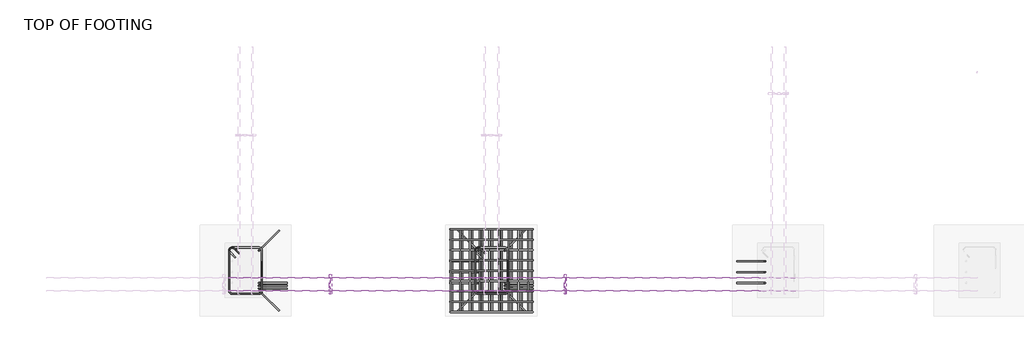
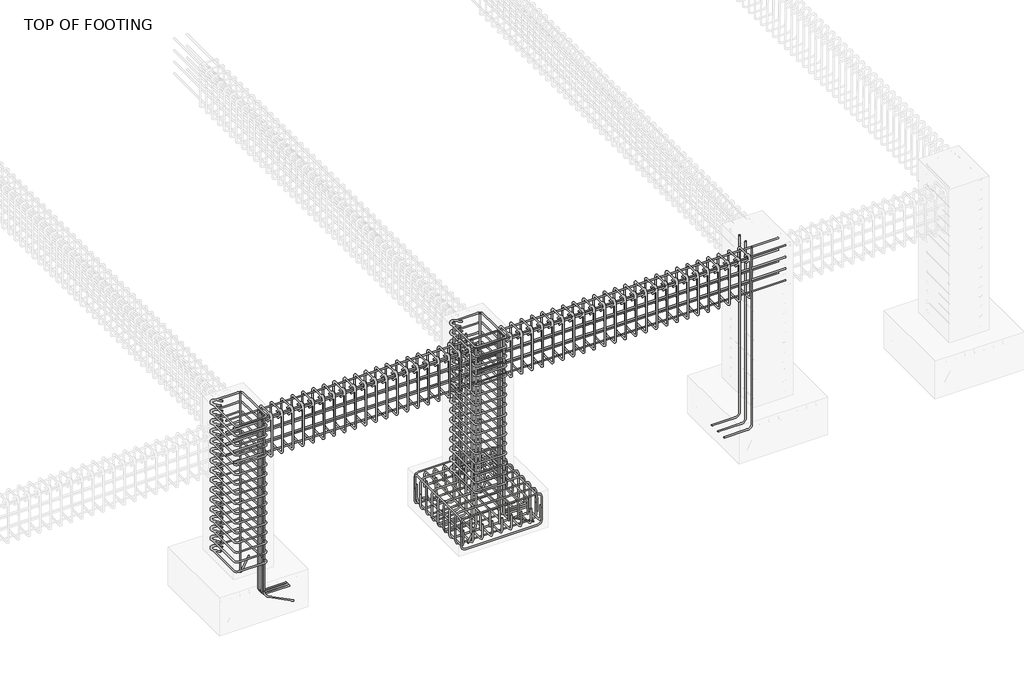
# One storey, part 3 of 9: 22 reinforcing bars.
"""IFC4 building model written with IfcOpenShell, lengths in millimetres."""

from ifc_helpers import new_model, si_unit, point, frame, origin, place, context, project, spatial, polyline, circle_curve, trimmed, segment, composite_curve, source, transform, mapped, element, save
from ifc_brep_helpers import swept_disk

model = new_model("IFC4")

# Units and contexts
model_context = context("Model", 3, world=origin())
ifc_project = project(units=[si_unit("LENGTHUNIT", "METRE", prefix="MILLI")], contexts=[model_context])

# Site, building, storey
site = spatial("IfcSite", under=ifc_project)
building = spatial("IfcBuilding", under=site)
storey = spatial("IfcBuildingStorey", under=building, Name="TOP OF FOOTING", Elevation=-1828.8)

# Reinforcing bars
placement = place(None, origin())
reinforcing_bar_shape = source(origin(), model_context, "Body", "SolidModel", [
    swept_disk(composite_curve([segment(polyline([(-4629.6174526, -598.6824927, -2052.8356656), (-4629.6174526, -598.6824927, -2200.1356656)]), True, "CONTINUOUS"), segment(trimmed(circle_curve(frame((-4675.9674526, -598.6824927, -2200.1356656), z_axis=(0.0, 1.0, 0.0), x_axis=(46.349999999999454, 0.0, 0.0)), 46.35), [point((-4629.6174526, -598.6824927, -2200.1356656))], [point((-4675.9674526, -598.6824927, -2246.4856656))], True, "CARTESIAN"), True, "CONTINUOUS"), segment(polyline([(-4675.9674526, -598.6824927, -2246.4856656), (-5490.5674526, -598.6824927, -2246.4856656)]), True, "CONTINUOUS"), segment(trimmed(circle_curve(frame((-5490.5674526, -598.6824927, -2200.1356656), z_axis=(0.0, 1.0, 0.0), x_axis=(0.0, 0.0, -46.350000000000364)), 46.35), [point((-5490.5674526, -598.6824927, -2246.4856656))], [point((-5536.9174526, -598.6824927, -2200.1356656))], True, "CARTESIAN"), True, "CONTINUOUS"), segment(polyline([(-5536.9174526, -598.6824927, -2200.1356656), (-5536.9174526, -598.6824927, -2052.8356656)]), True, "CONTINUOUS")], self_intersect=False), 6.35),
])
element("IfcReinforcingBar", 1, at=placement, inside=storey, context=model_context, shape_type="MappedRepresentation", body=[
    mapped(reinforcing_bar_shape, transform((0.0, 0.0, 0.0), x_axis=(1.0, 0.0, 0.0), y_axis=(0.0, 1.0, 0.0), z_axis=(0.0, 0.0, 1.0))),
    mapped(reinforcing_bar_shape, transform((0.0, -113.4125, 0.0), x_axis=(1.0, 0.0, 0.0), y_axis=(0.0, 1.0, 0.0), z_axis=(0.0, 0.0, 1.0))),
    mapped(reinforcing_bar_shape, transform((0.0, -226.825, 0.0), x_axis=(1.0, 0.0, 0.0), y_axis=(0.0, 1.0, 0.0), z_axis=(0.0, 0.0, 1.0))),
    mapped(reinforcing_bar_shape, transform((0.0, -340.2375, 0.0), x_axis=(1.0, 0.0, 0.0), y_axis=(0.0, 1.0, 0.0), z_axis=(0.0, 0.0, 1.0))),
    mapped(reinforcing_bar_shape, transform((0.0, -453.65, 0.0), x_axis=(1.0, 0.0, 0.0), y_axis=(0.0, 1.0, 0.0), z_axis=(0.0, 0.0, 1.0))),
    mapped(reinforcing_bar_shape, transform((0.0, -567.0625, 0.0), x_axis=(1.0, 0.0, 0.0), y_axis=(0.0, 1.0, 0.0), z_axis=(0.0, 0.0, 1.0))),
    mapped(reinforcing_bar_shape, transform((0.0, -680.475, 0.0), x_axis=(1.0, 0.0, 0.0), y_axis=(0.0, 1.0, 0.0), z_axis=(0.0, 0.0, 1.0))),
    mapped(reinforcing_bar_shape, transform((0.0, -793.8875, 0.0), x_axis=(1.0, 0.0, 0.0), y_axis=(0.0, 1.0, 0.0), z_axis=(0.0, 0.0, 1.0))),
    mapped(reinforcing_bar_shape, transform((0.0, -907.3, 0.0), x_axis=(1.0, 0.0, 0.0), y_axis=(0.0, 1.0, 0.0), z_axis=(0.0, 0.0, 1.0))),
])
reinforcing_bar_2_shape = source(origin(), model_context, "Body", "SolidModel", [
    swept_disk(composite_curve([segment(polyline([(-5536.9174526, -598.6824927, -2068.8), (-5536.9174526, -598.6824927, -1921.5)]), True, "CONTINUOUS"), segment(trimmed(circle_curve(frame((-5490.5674526, -598.6824927, -1921.5), z_axis=(0.0, 1.0, 0.0), x_axis=(-46.349999999999454, 0.0, 0.0)), 46.35), [point((-5536.9174526, -598.6824927, -1921.5))], [point((-5490.5674526, -598.6824927, -1875.15))], True, "CARTESIAN"), True, "CONTINUOUS"), segment(polyline([(-5490.5674526, -598.6824927, -1875.15), (-4675.9674526, -598.6824927, -1875.15)]), True, "CONTINUOUS"), segment(trimmed(circle_curve(frame((-4675.9674526, -598.6824927, -1921.5), z_axis=(0.0, 1.0, 0.0), x_axis=(0.0, 0.0, 46.34999999999991)), 46.35), [point((-4675.9674526, -598.6824927, -1875.15))], [point((-4629.6174526, -598.6824927, -1921.5))], True, "CARTESIAN"), True, "CONTINUOUS"), segment(polyline([(-4629.6174526, -598.6824927, -1921.5), (-4629.6174526, -598.6824927, -2068.8)]), True, "CONTINUOUS")], self_intersect=False), 6.35),
])
element("IfcReinforcingBar", 2, at=placement, inside=storey, context=model_context, shape_type="MappedRepresentation", body=[
    mapped(reinforcing_bar_2_shape, transform((0.0, 0.0, 0.0), x_axis=(1.0, 0.0, 0.0), y_axis=(0.0, 1.0, 0.0), z_axis=(0.0, 0.0, 1.0))),
    mapped(reinforcing_bar_2_shape, transform((0.0, -113.4125, 0.0), x_axis=(1.0, 0.0, 0.0), y_axis=(0.0, 1.0, 0.0), z_axis=(0.0, 0.0, 1.0))),
    mapped(reinforcing_bar_2_shape, transform((0.0, -226.825, 0.0), x_axis=(1.0, 0.0, 0.0), y_axis=(0.0, 1.0, 0.0), z_axis=(0.0, 0.0, 1.0))),
    mapped(reinforcing_bar_2_shape, transform((0.0, -340.2375, 0.0), x_axis=(1.0, 0.0, 0.0), y_axis=(0.0, 1.0, 0.0), z_axis=(0.0, 0.0, 1.0))),
    mapped(reinforcing_bar_2_shape, transform((0.0, -453.65, 0.0), x_axis=(1.0, 0.0, 0.0), y_axis=(0.0, 1.0, 0.0), z_axis=(0.0, 0.0, 1.0))),
    mapped(reinforcing_bar_2_shape, transform((0.0, -567.0625, 0.0), x_axis=(1.0, 0.0, 0.0), y_axis=(0.0, 1.0, 0.0), z_axis=(0.0, 0.0, 1.0))),
    mapped(reinforcing_bar_2_shape, transform((0.0, -680.475, 0.0), x_axis=(1.0, 0.0, 0.0), y_axis=(0.0, 1.0, 0.0), z_axis=(0.0, 0.0, 1.0))),
    mapped(reinforcing_bar_2_shape, transform((0.0, -793.8875, 0.0), x_axis=(1.0, 0.0, 0.0), y_axis=(0.0, 1.0, 0.0), z_axis=(0.0, 0.0, 1.0))),
    mapped(reinforcing_bar_2_shape, transform((0.0, -907.3, 0.0), x_axis=(1.0, 0.0, 0.0), y_axis=(0.0, 1.0, 0.0), z_axis=(0.0, 0.0, 1.0))),
])
reinforcing_bar_3_shape = source(origin(), model_context, "Body", "SolidModel", [
    swept_disk(composite_curve([segment(polyline([(-5513.2674526, -598.6824927, -2020.15), (-5513.2674526, -598.6824927, -2167.45)]), True, "CONTINUOUS"), segment(trimmed(circle_curve(frame((-5513.2674526, -645.0324927, -2167.45), z_axis=(-1.0, 0.0, 0.0), x_axis=(0.0, 46.35000000000002, 0.0)), 46.35), [point((-5513.2674526, -598.6824927, -2167.45))], [point((-5513.2674526, -645.0324927, -2213.8))], True, "CARTESIAN"), True, "CONTINUOUS"), segment(polyline([(-5513.2674526, -645.0324927, -2213.8), (-5513.2674526, -1459.6324927, -2213.8)]), True, "CONTINUOUS"), segment(trimmed(circle_curve(frame((-5513.2674526, -1459.6324927, -2167.45), z_axis=(-1.0, 0.0, 0.0), x_axis=(0.0, 0.0, -46.350000000000364)), 46.35), [point((-5513.2674526, -1459.6324927, -2213.8))], [point((-5513.2674526, -1505.9824927, -2167.45))], True, "CARTESIAN"), True, "CONTINUOUS"), segment(polyline([(-5513.2674526, -1505.9824927, -2167.45), (-5513.2674526, -1505.9824927, -2020.15)]), True, "CONTINUOUS")], self_intersect=False), 6.35),
])
element("IfcReinforcingBar", 3, at=placement, inside=storey, context=model_context, shape_type="MappedRepresentation", body=[
    mapped(reinforcing_bar_3_shape, transform((0.0, 0.0, 0.0), x_axis=(1.0, 0.0, 0.0), y_axis=(0.0, 1.0, 0.0), z_axis=(0.0, 0.0, 1.0))),
    mapped(reinforcing_bar_3_shape, transform((108.8370374, 0.0, 0.0), x_axis=(1.0, 0.0, 0.0), y_axis=(0.0, 1.0, 0.0), z_axis=(0.0, 0.0, 1.0))),
    mapped(reinforcing_bar_3_shape, transform((217.6740748, 0.0, 0.0), x_axis=(1.0, 0.0, 0.0), y_axis=(0.0, 1.0, 0.0), z_axis=(0.0, 0.0, 1.0))),
    mapped(reinforcing_bar_3_shape, transform((326.5111123, 0.0, 0.0), x_axis=(1.0, 0.0, 0.0), y_axis=(0.0, 1.0, 0.0), z_axis=(0.0, 0.0, 1.0))),
    mapped(reinforcing_bar_3_shape, transform((435.3481497, 0.0, 0.0), x_axis=(1.0, 0.0, 0.0), y_axis=(0.0, 1.0, 0.0), z_axis=(0.0, 0.0, 1.0))),
    mapped(reinforcing_bar_3_shape, transform((544.1851871, 0.0, 0.0), x_axis=(1.0, 0.0, 0.0), y_axis=(0.0, 1.0, 0.0), z_axis=(0.0, 0.0, 1.0))),
    mapped(reinforcing_bar_3_shape, transform((653.0222245, 0.0, 0.0), x_axis=(1.0, 0.0, 0.0), y_axis=(0.0, 1.0, 0.0), z_axis=(0.0, 0.0, 1.0))),
    mapped(reinforcing_bar_3_shape, transform((761.8592619, 0.0, 0.0), x_axis=(1.0, 0.0, 0.0), y_axis=(0.0, 1.0, 0.0), z_axis=(0.0, 0.0, 1.0))),
    mapped(reinforcing_bar_3_shape, transform((870.6962994, 0.0, 0.0), x_axis=(1.0, 0.0, 0.0), y_axis=(0.0, 1.0, 0.0), z_axis=(0.0, 0.0, 1.0))),
])
reinforcing_bar_4_shape = source(origin(), model_context, "Body", "SolidModel", [
    swept_disk(composite_curve([segment(polyline([(-4680.7455787, -598.6824927, -2076.9782245), (-4680.7455787, -598.6824927, -1929.6782245)]), True, "CONTINUOUS"), segment(trimmed(circle_curve(frame((-4680.7455787, -645.0324927, -1929.6782245), z_axis=(1.0, 0.0, 0.0), x_axis=(0.0, 46.35000000000002, 0.0)), 46.35), [point((-4680.7455787, -598.6824927, -1929.6782245))], [point((-4680.7455787, -645.0324927, -1883.3282245))], True, "CARTESIAN"), True, "CONTINUOUS"), segment(polyline([(-4680.7455787, -645.0324927, -1883.3282245), (-4680.7455787, -1459.6324927, -1883.3282245)]), True, "CONTINUOUS"), segment(trimmed(circle_curve(frame((-4680.7455787, -1459.6324927, -1929.6782245), z_axis=(1.0, 0.0, 0.0), x_axis=(0.0, 0.0, 46.34999999999991)), 46.35), [point((-4680.7455787, -1459.6324927, -1883.3282245))], [point((-4680.7455787, -1505.9824927, -1929.6782245))], True, "CARTESIAN"), True, "CONTINUOUS"), segment(polyline([(-4680.7455787, -1505.9824927, -1929.6782245), (-4680.7455787, -1505.9824927, -2076.9782245)]), True, "CONTINUOUS")], self_intersect=False), 6.35),
])
element("IfcReinforcingBar", 4, at=placement, inside=storey, context=model_context, shape_type="MappedRepresentation", body=[
    mapped(reinforcing_bar_4_shape, transform((0.0, 0.0, 0.0), x_axis=(1.0, 0.0, 0.0), y_axis=(0.0, 1.0, 0.0), z_axis=(0.0, 0.0, 1.0))),
    mapped(reinforcing_bar_4_shape, transform((-106.3275638, 0.0, 0.0), x_axis=(1.0, 0.0, 0.0), y_axis=(0.0, 1.0, 0.0), z_axis=(0.0, 0.0, 1.0))),
    mapped(reinforcing_bar_4_shape, transform((-212.6551275, 0.0, 0.0), x_axis=(1.0, 0.0, 0.0), y_axis=(0.0, 1.0, 0.0), z_axis=(0.0, 0.0, 1.0))),
    mapped(reinforcing_bar_4_shape, transform((-318.9826913, 0.0, 0.0), x_axis=(1.0, 0.0, 0.0), y_axis=(0.0, 1.0, 0.0), z_axis=(0.0, 0.0, 1.0))),
    mapped(reinforcing_bar_4_shape, transform((-425.310255, 0.0, 0.0), x_axis=(1.0, 0.0, 0.0), y_axis=(0.0, 1.0, 0.0), z_axis=(0.0, 0.0, 1.0))),
    mapped(reinforcing_bar_4_shape, transform((-531.6378188, 0.0, 0.0), x_axis=(1.0, 0.0, 0.0), y_axis=(0.0, 1.0, 0.0), z_axis=(0.0, 0.0, 1.0))),
    mapped(reinforcing_bar_4_shape, transform((-637.9653825, 0.0, 0.0), x_axis=(1.0, 0.0, 0.0), y_axis=(0.0, 1.0, 0.0), z_axis=(0.0, 0.0, 1.0))),
    mapped(reinforcing_bar_4_shape, transform((-744.2929463, 0.0, 0.0), x_axis=(1.0, 0.0, 0.0), y_axis=(0.0, 1.0, 0.0), z_axis=(0.0, 0.0, 1.0))),
    mapped(reinforcing_bar_4_shape, transform((-850.62051, 0.0, 0.0), x_axis=(1.0, 0.0, 0.0), y_axis=(0.0, 1.0, 0.0), z_axis=(0.0, 0.0, 1.0))),
])
reinforcing_bar_5_shape = source(origin(), model_context, "Body", "SolidModel", [
    swept_disk(composite_curve([segment(polyline([(-7852.6560921, -863.6082581, -1782.45), (-7908.399655, -807.8646951, -1782.45)]), True, "CONTINUOUS"), segment(trimmed(circle_curve(frame((-7930.5674526, -830.0324927, -1782.45), z_axis=(0.0, 0.0, 1.0), x_axis=(22.167797600000085, 22.167797600000085, 0.0)), 31.35), [point((-7908.399655, -807.8646951, -1782.45))], [point((-7961.9174526, -830.0324927, -1782.45))], True, "CARTESIAN"), True, "CONTINUOUS"), segment(polyline([(-7961.9174526, -830.0324927, -1782.45), (-7961.9174526, -1274.6324927, -1782.45)]), True, "CONTINUOUS"), segment(trimmed(circle_curve(frame((-7930.5674526, -1274.6324927, -1782.45), z_axis=(0.0, 0.0, 1.0), x_axis=(-31.349999999999454, 0.0, 0.0)), 31.35), [point((-7961.9174526, -1274.6324927, -1782.45))], [point((-7930.5674526, -1305.9824927, -1782.45))], True, "CARTESIAN"), True, "CONTINUOUS"), segment(polyline([(-7930.5674526, -1305.9824927, -1782.45), (-7635.9674526, -1305.9824927, -1782.45)]), True, "CONTINUOUS"), segment(trimmed(circle_curve(frame((-7635.9674526, -1274.642312, -1783.2345856), z_axis=(0.0, 0.025026655153786315, 0.9996867842138424), x_axis=(0.0, -31.34018070000002, 0.7845855999999003)), 31.35), [point((-7635.9674526, -1305.9824927, -1782.45))], [point((-7604.6174526, -1274.642312, -1783.2345856))], True, "CARTESIAN"), True, "CONTINUOUS"), segment(polyline([(-7604.6174526, -1274.642312, -1783.2345856), (-7604.6174526, -830.0226734, -1794.3654144)]), True, "CONTINUOUS"), segment(trimmed(circle_curve(frame((-7635.9674526, -830.0226734, -1794.3654144), z_axis=(0.0, 0.025026655153786315, 0.9996867842138424), x_axis=(31.349999999999454, 0.0, 0.0)), 31.35), [point((-7604.6174526, -830.0226734, -1794.3654144))], [point((-7635.9674526, -798.6824927, -1795.15))], True, "CARTESIAN"), True, "CONTINUOUS"), segment(polyline([(-7635.9674526, -798.6824927, -1795.15), (-7930.5674526, -798.6824927, -1795.15)]), True, "CONTINUOUS"), segment(trimmed(circle_curve(frame((-7930.5674526, -830.0324927, -1795.15), z_axis=(0.0, 0.0, 1.0), x_axis=(0.0, 31.350000000000023, 0.0)), 31.35), [point((-7930.5674526, -798.6824927, -1795.15))], [point((-7952.7352502, -852.2002903, -1795.15))], True, "CARTESIAN"), True, "CONTINUOUS"), segment(polyline([(-7952.7352502, -852.2002903, -1795.15), (-7896.9916873, -907.9438533, -1795.15)]), True, "CONTINUOUS")], self_intersect=False), 6.35),
])
element("IfcReinforcingBar", 5, at=placement, inside=storey, context=model_context, shape_type="MappedRepresentation", body=[
    mapped(reinforcing_bar_5_shape, transform((0.0, 0.0, 0.0), x_axis=(1.0, 0.0, 0.0), y_axis=(0.0, 1.0, 0.0), z_axis=(0.0, 0.0, 1.0))),
    mapped(reinforcing_bar_5_shape, transform((0.0, 0.0, 115.74), x_axis=(1.0, 0.0, 0.0), y_axis=(0.0, 1.0, 0.0), z_axis=(0.0, 0.0, 1.0))),
    mapped(reinforcing_bar_5_shape, transform((0.0, 0.0, 231.48), x_axis=(1.0, 0.0, 0.0), y_axis=(0.0, 1.0, 0.0), z_axis=(0.0, 0.0, 1.0))),
    mapped(reinforcing_bar_5_shape, transform((0.0, 0.0, 347.22), x_axis=(1.0, 0.0, 0.0), y_axis=(0.0, 1.0, 0.0), z_axis=(0.0, 0.0, 1.0))),
    mapped(reinforcing_bar_5_shape, transform((0.0, 0.0, 462.96), x_axis=(1.0, 0.0, 0.0), y_axis=(0.0, 1.0, 0.0), z_axis=(0.0, 0.0, 1.0))),
    mapped(reinforcing_bar_5_shape, transform((0.0, 0.0, 578.7), x_axis=(1.0, 0.0, 0.0), y_axis=(0.0, 1.0, 0.0), z_axis=(0.0, 0.0, 1.0))),
    mapped(reinforcing_bar_5_shape, transform((0.0, 0.0, 694.44), x_axis=(1.0, 0.0, 0.0), y_axis=(0.0, 1.0, 0.0), z_axis=(0.0, 0.0, 1.0))),
    mapped(reinforcing_bar_5_shape, transform((0.0, 0.0, 810.18), x_axis=(1.0, 0.0, 0.0), y_axis=(0.0, 1.0, 0.0), z_axis=(0.0, 0.0, 1.0))),
    mapped(reinforcing_bar_5_shape, transform((0.0, 0.0, 925.92), x_axis=(1.0, 0.0, 0.0), y_axis=(0.0, 1.0, 0.0), z_axis=(0.0, 0.0, 1.0))),
    mapped(reinforcing_bar_5_shape, transform((0.0, 0.0, 1041.66), x_axis=(1.0, 0.0, 0.0), y_axis=(0.0, 1.0, 0.0), z_axis=(0.0, 0.0, 1.0))),
    mapped(reinforcing_bar_5_shape, transform((0.0, 0.0, 1157.4), x_axis=(1.0, 0.0, 0.0), y_axis=(0.0, 1.0, 0.0), z_axis=(0.0, 0.0, 1.0))),
    mapped(reinforcing_bar_5_shape, transform((0.0, 0.0, 1273.14), x_axis=(1.0, 0.0, 0.0), y_axis=(0.0, 1.0, 0.0), z_axis=(0.0, 0.0, 1.0))),
    mapped(reinforcing_bar_5_shape, transform((0.0, 0.0, 1388.88), x_axis=(1.0, 0.0, 0.0), y_axis=(0.0, 1.0, 0.0), z_axis=(0.0, 0.0, 1.0))),
    mapped(reinforcing_bar_5_shape, transform((0.0, 0.0, 1504.62), x_axis=(1.0, 0.0, 0.0), y_axis=(0.0, 1.0, 0.0), z_axis=(0.0, 0.0, 1.0))),
    mapped(reinforcing_bar_5_shape, transform((0.0, 0.0, 1620.36), x_axis=(1.0, 0.0, 0.0), y_axis=(0.0, 1.0, 0.0), z_axis=(0.0, 0.0, 1.0))),
    mapped(reinforcing_bar_5_shape, transform((0.0, 0.0, 1736.1), x_axis=(1.0, 0.0, 0.0), y_axis=(0.0, 1.0, 0.0), z_axis=(0.0, 0.0, 1.0))),
])
element("IfcReinforcingBar", 6, at=placement, inside=storey, context=model_context, shape_type="SolidModel", body=[
    swept_disk(composite_curve([segment(polyline([(-7635.9674526, -832.8986176, -40.0), (-7635.9674526, -832.8986176, -2148.1729582)]), True, "CONTINUOUS"), segment(trimmed(circle_curve(frame((-7603.1930533, -800.1242183, -2148.1729582), z_axis=(0.7071067811865507, -0.7071067811865444, 0.0), x_axis=(-32.77439929999946, -32.774399299999914, 0.0)), 46.35), [point((-7635.9674526, -832.8986176, -2148.1729582))], [point((-7603.1930533, -800.1242183, -2194.5229582))], True, "CARTESIAN"), True, "CONTINUOUS"), segment(polyline([(-7603.1930533, -800.1242183, -2194.5229582), (-7414.6811959, -611.6123609, -2194.5229582)]), True, "CONTINUOUS")], self_intersect=False), 6.35),
])
element("IfcReinforcingBar", 7, at=placement, inside=storey, context=model_context, shape_type="SolidModel", body=[
    swept_disk(composite_curve([segment(polyline([(-7626.0216728, -1281.7121476, -40.0), (-7626.0216728, -1281.7121476, -2148.1729582)]), True, "CONTINUOUS"), segment(trimmed(circle_curve(frame((-7593.2472735, -1314.4865469, -2148.1729582), z_axis=(-0.707106781186547, -0.707106781186548, 0.0), x_axis=(-32.77439929999946, 32.774399299999914, 0.0)), 46.35), [point((-7626.0216728, -1281.7121476, -2148.1729582))], [point((-7593.2472735, -1314.4865469, -2194.5229582))], True, "CARTESIAN"), True, "CONTINUOUS"), segment(polyline([(-7593.2472735, -1314.4865469, -2194.5229582), (-7414.6811959, -1493.0526245, -2194.5229582)]), True, "CONTINUOUS")], self_intersect=False), 6.35),
])
reinforcing_bar_6_shape = source(origin(), model_context, "Body", "SolidModel", [
    swept_disk(composite_curve([segment(polyline([(-7635.9674526, -1187.8357134, -40.0), (-7635.9674526, -1187.8357134, -2148.1729582)]), True, "CONTINUOUS"), segment(trimmed(circle_curve(frame((-7589.6174526, -1187.8357134, -2148.1729582), z_axis=(0.0, -1.0, 0.0), x_axis=(-46.349999999999454, 0.0, 0.0)), 46.35), [point((-7635.9674526, -1187.8357134, -2148.1729582))], [point((-7589.6174526, -1187.8357134, -2194.5229582))], True, "CARTESIAN"), True, "CONTINUOUS"), segment(polyline([(-7589.6174526, -1187.8357134, -2194.5229582), (-7323.0214272, -1187.8357134, -2194.5229582)]), True, "CONTINUOUS")], self_intersect=False), 6.35),
])
element("IfcReinforcingBar", 8, at=placement, inside=storey, context=model_context, shape_type="MappedRepresentation", body=[
    mapped(reinforcing_bar_6_shape, transform((0.0, 0.0, 0.0), x_axis=(1.0, 0.0, 0.0), y_axis=(0.0, 1.0, 0.0), z_axis=(0.0, 0.0, 1.0))),
    mapped(reinforcing_bar_6_shape, transform((0.0, -30.8635533, 0.0), x_axis=(1.0, 0.0, 0.0), y_axis=(0.0, 1.0, 0.0), z_axis=(0.0, 0.0, 1.0))),
    mapped(reinforcing_bar_6_shape, transform((0.0, -61.7271066, 0.0), x_axis=(1.0, 0.0, 0.0), y_axis=(0.0, 1.0, 0.0), z_axis=(0.0, 0.0, 1.0))),
])
reinforcing_bar_7_shape = source(origin(), model_context, "Body", "SolidModel", [
    swept_disk(composite_curve([segment(polyline([(-5230.5674526, -1187.8357134, -40.0), (-5230.5674526, -1187.8357134, -2148.1729582)]), True, "CONTINUOUS"), segment(trimmed(circle_curve(frame((-5276.9174526, -1187.8357134, -2148.1729582), z_axis=(0.0, 1.0, 0.0), x_axis=(46.349999999999454, 0.0, 0.0)), 46.35), [point((-5230.5674526, -1187.8357134, -2148.1729582))], [point((-5276.9174526, -1187.8357134, -2194.5229582))], True, "CARTESIAN"), True, "CONTINUOUS"), segment(polyline([(-5276.9174526, -1187.8357134, -2194.5229582), (-5543.513478, -1187.8357134, -2194.5229582)]), True, "CONTINUOUS")], self_intersect=False), 6.35),
])
element("IfcReinforcingBar", 9, at=placement, inside=storey, context=model_context, shape_type="MappedRepresentation", body=[
    mapped(reinforcing_bar_7_shape, transform((0.0, 0.0, 0.0), x_axis=(1.0, 0.0, 0.0), y_axis=(0.0, 1.0, 0.0), z_axis=(0.0, 0.0, 1.0))),
    mapped(reinforcing_bar_7_shape, transform((0.0, 119.1364467, 0.0), x_axis=(1.0, 0.0, 0.0), y_axis=(0.0, 1.0, 0.0), z_axis=(0.0, 0.0, 1.0))),
    mapped(reinforcing_bar_7_shape, transform((0.0, 238.2728934, 0.0), x_axis=(1.0, 0.0, 0.0), y_axis=(0.0, 1.0, 0.0), z_axis=(0.0, 0.0, 1.0))),
])
reinforcing_bar_8_shape = source(origin(), model_context, "Body", "SolidModel", [
    swept_disk(composite_curve([segment(polyline([(-5152.6560921, -863.6082581, -1782.45), (-5208.399655, -807.8646951, -1782.45)]), True, "CONTINUOUS"), segment(trimmed(circle_curve(frame((-5230.5674526, -830.0324927, -1782.45), z_axis=(0.0, 0.0, 1.0), x_axis=(22.167797600000085, 22.167797600000085, 0.0)), 31.35), [point((-5208.399655, -807.8646951, -1782.45))], [point((-5261.9174526, -830.0324927, -1782.45))], True, "CARTESIAN"), True, "CONTINUOUS"), segment(polyline([(-5261.9174526, -830.0324927, -1782.45), (-5261.9174526, -1274.6324927, -1782.45)]), True, "CONTINUOUS"), segment(trimmed(circle_curve(frame((-5230.5674526, -1274.6324927, -1782.45), z_axis=(0.0, 0.0, 1.0), x_axis=(-31.349999999999454, 0.0, 0.0)), 31.35), [point((-5261.9174526, -1274.6324927, -1782.45))], [point((-5230.5674526, -1305.9824927, -1782.45))], True, "CARTESIAN"), True, "CONTINUOUS"), segment(polyline([(-5230.5674526, -1305.9824927, -1782.45), (-4935.9674526, -1305.9824927, -1782.45)]), True, "CONTINUOUS"), segment(trimmed(circle_curve(frame((-4935.9674526, -1274.642312, -1783.2345856), z_axis=(0.0, 0.025026655153786315, 0.9996867842138424), x_axis=(0.0, -31.34018070000002, 0.7845855999999003)), 31.35), [point((-4935.9674526, -1305.9824927, -1782.45))], [point((-4904.6174526, -1274.642312, -1783.2345856))], True, "CARTESIAN"), True, "CONTINUOUS"), segment(polyline([(-4904.6174526, -1274.642312, -1783.2345856), (-4904.6174526, -830.0226734, -1794.3654144)]), True, "CONTINUOUS"), segment(trimmed(circle_curve(frame((-4935.9674526, -830.0226734, -1794.3654144), z_axis=(0.0, 0.025026655153786315, 0.9996867842138424), x_axis=(31.349999999999454, 0.0, 0.0)), 31.35), [point((-4904.6174526, -830.0226734, -1794.3654144))], [point((-4935.9674526, -798.6824927, -1795.15))], True, "CARTESIAN"), True, "CONTINUOUS"), segment(polyline([(-4935.9674526, -798.6824927, -1795.15), (-5230.5674526, -798.6824927, -1795.15)]), True, "CONTINUOUS"), segment(trimmed(circle_curve(frame((-5230.5674526, -830.0324927, -1795.15), z_axis=(0.0, 0.0, 1.0), x_axis=(0.0, 31.350000000000023, 0.0)), 31.35), [point((-5230.5674526, -798.6824927, -1795.15))], [point((-5252.7352502, -852.2002903, -1795.15))], True, "CARTESIAN"), True, "CONTINUOUS"), segment(polyline([(-5252.7352502, -852.2002903, -1795.15), (-5196.9916873, -907.9438533, -1795.15)]), True, "CONTINUOUS")], self_intersect=False), 6.35),
])
element("IfcReinforcingBar", 10, at=placement, inside=storey, context=model_context, shape_type="MappedRepresentation", body=[
    mapped(reinforcing_bar_8_shape, transform((0.0, 0.0, 0.0), x_axis=(1.0, 0.0, 0.0), y_axis=(0.0, 1.0, 0.0), z_axis=(0.0, 0.0, 1.0))),
    mapped(reinforcing_bar_8_shape, transform((0.0, 0.0, 115.74), x_axis=(1.0, 0.0, 0.0), y_axis=(0.0, 1.0, 0.0), z_axis=(0.0, 0.0, 1.0))),
    mapped(reinforcing_bar_8_shape, transform((0.0, 0.0, 231.48), x_axis=(1.0, 0.0, 0.0), y_axis=(0.0, 1.0, 0.0), z_axis=(0.0, 0.0, 1.0))),
    mapped(reinforcing_bar_8_shape, transform((0.0, 0.0, 347.22), x_axis=(1.0, 0.0, 0.0), y_axis=(0.0, 1.0, 0.0), z_axis=(0.0, 0.0, 1.0))),
    mapped(reinforcing_bar_8_shape, transform((0.0, 0.0, 462.96), x_axis=(1.0, 0.0, 0.0), y_axis=(0.0, 1.0, 0.0), z_axis=(0.0, 0.0, 1.0))),
    mapped(reinforcing_bar_8_shape, transform((0.0, 0.0, 578.7), x_axis=(1.0, 0.0, 0.0), y_axis=(0.0, 1.0, 0.0), z_axis=(0.0, 0.0, 1.0))),
    mapped(reinforcing_bar_8_shape, transform((0.0, 0.0, 694.44), x_axis=(1.0, 0.0, 0.0), y_axis=(0.0, 1.0, 0.0), z_axis=(0.0, 0.0, 1.0))),
    mapped(reinforcing_bar_8_shape, transform((0.0, 0.0, 810.18), x_axis=(1.0, 0.0, 0.0), y_axis=(0.0, 1.0, 0.0), z_axis=(0.0, 0.0, 1.0))),
    mapped(reinforcing_bar_8_shape, transform((0.0, 0.0, 925.92), x_axis=(1.0, 0.0, 0.0), y_axis=(0.0, 1.0, 0.0), z_axis=(0.0, 0.0, 1.0))),
    mapped(reinforcing_bar_8_shape, transform((0.0, 0.0, 1041.66), x_axis=(1.0, 0.0, 0.0), y_axis=(0.0, 1.0, 0.0), z_axis=(0.0, 0.0, 1.0))),
    mapped(reinforcing_bar_8_shape, transform((0.0, 0.0, 1157.4), x_axis=(1.0, 0.0, 0.0), y_axis=(0.0, 1.0, 0.0), z_axis=(0.0, 0.0, 1.0))),
    mapped(reinforcing_bar_8_shape, transform((0.0, 0.0, 1273.14), x_axis=(1.0, 0.0, 0.0), y_axis=(0.0, 1.0, 0.0), z_axis=(0.0, 0.0, 1.0))),
    mapped(reinforcing_bar_8_shape, transform((0.0, 0.0, 1388.88), x_axis=(1.0, 0.0, 0.0), y_axis=(0.0, 1.0, 0.0), z_axis=(0.0, 0.0, 1.0))),
    mapped(reinforcing_bar_8_shape, transform((0.0, 0.0, 1504.62), x_axis=(1.0, 0.0, 0.0), y_axis=(0.0, 1.0, 0.0), z_axis=(0.0, 0.0, 1.0))),
    mapped(reinforcing_bar_8_shape, transform((0.0, 0.0, 1620.36), x_axis=(1.0, 0.0, 0.0), y_axis=(0.0, 1.0, 0.0), z_axis=(0.0, 0.0, 1.0))),
    mapped(reinforcing_bar_8_shape, transform((0.0, 0.0, 1736.1), x_axis=(1.0, 0.0, 0.0), y_axis=(0.0, 1.0, 0.0), z_axis=(0.0, 0.0, 1.0))),
])
element("IfcReinforcingBar", 11, at=placement, inside=storey, context=model_context, shape_type="SolidModel", body=[
    swept_disk(composite_curve([segment(polyline([(-5230.5674526, -832.8986176, -40.0), (-5230.5674526, -832.8986176, -2148.1729582)]), True, "CONTINUOUS"), segment(trimmed(circle_curve(frame((-5263.3418519, -800.1242183, -2148.1729582), z_axis=(0.7071067811865507, 0.7071067811865444, 0.0), x_axis=(32.77439929999946, -32.774399299999914, 0.0)), 46.35), [point((-5230.5674526, -832.8986176, -2148.1729582))], [point((-5263.3418519, -800.1242183, -2194.5229582))], True, "CARTESIAN"), True, "CONTINUOUS"), segment(polyline([(-5263.3418519, -800.1242183, -2194.5229582), (-5451.8537093, -611.6123609, -2194.5229582)]), True, "CONTINUOUS")], self_intersect=False), 6.35),
])
element("IfcReinforcingBar", 12, at=placement, inside=storey, context=model_context, shape_type="SolidModel", body=[
    swept_disk(composite_curve([segment(polyline([(-5240.5132324, -1281.7121476, -40.0), (-5240.5132324, -1281.7121476, -2148.1729582)]), True, "CONTINUOUS"), segment(trimmed(circle_curve(frame((-5273.2876317, -1314.4865469, -2148.1729582), z_axis=(-0.707106781186547, 0.707106781186548, 0.0), x_axis=(32.77439930000037, 32.774399299999914, 0.0)), 46.35), [point((-5240.5132324, -1281.7121476, -2148.1729582))], [point((-5273.2876317, -1314.4865469, -2194.5229582))], True, "CARTESIAN"), True, "CONTINUOUS"), segment(polyline([(-5273.2876317, -1314.4865469, -2194.5229582), (-5451.8537093, -1493.0526245, -2194.5229582)]), True, "CONTINUOUS")], self_intersect=False), 6.35),
])
element("IfcReinforcingBar", 13, at=placement, inside=storey, context=model_context, shape_type="SolidModel", body=[
    swept_disk(composite_curve([segment(polyline([(-4935.9674526, -832.8986176, -40.0), (-4935.9674526, -832.8986176, -2148.1729582)]), True, "CONTINUOUS"), segment(trimmed(circle_curve(frame((-4903.1930533, -800.1242183, -2148.1729582), z_axis=(0.7071067811865507, -0.7071067811865444, 0.0), x_axis=(-32.77439929999946, -32.774399299999914, 0.0)), 46.35), [point((-4935.9674526, -832.8986176, -2148.1729582))], [point((-4903.1930533, -800.1242183, -2194.5229582))], True, "CARTESIAN"), True, "CONTINUOUS"), segment(polyline([(-4903.1930533, -800.1242183, -2194.5229582), (-4714.6811959, -611.6123609, -2194.5229582)]), True, "CONTINUOUS")], self_intersect=False), 6.35),
])
element("IfcReinforcingBar", 14, at=placement, inside=storey, context=model_context, shape_type="SolidModel", body=[
    swept_disk(composite_curve([segment(polyline([(-4926.0216728, -1281.7121476, -40.0), (-4926.0216728, -1281.7121476, -2148.1729582)]), True, "CONTINUOUS"), segment(trimmed(circle_curve(frame((-4893.2472735, -1314.4865469, -2148.1729582), z_axis=(-0.707106781186547, -0.707106781186548, 0.0), x_axis=(-32.77439929999946, 32.774399299999914, 0.0)), 46.35), [point((-4926.0216728, -1281.7121476, -2148.1729582))], [point((-4893.2472735, -1314.4865469, -2194.5229582))], True, "CARTESIAN"), True, "CONTINUOUS"), segment(polyline([(-4893.2472735, -1314.4865469, -2194.5229582), (-4714.6811959, -1493.0526245, -2194.5229582)]), True, "CONTINUOUS")], self_intersect=False), 6.35),
])
reinforcing_bar_9_shape = source(origin(), model_context, "Body", "SolidModel", [
    swept_disk(composite_curve([segment(polyline([(-4935.9674526, -1187.8357134, -40.0), (-4935.9674526, -1187.8357134, -2148.1729582)]), True, "CONTINUOUS"), segment(trimmed(circle_curve(frame((-4889.6174526, -1187.8357134, -2148.1729582), z_axis=(0.0, -1.0, 0.0), x_axis=(-46.349999999999454, 0.0, 0.0)), 46.35), [point((-4935.9674526, -1187.8357134, -2148.1729582))], [point((-4889.6174526, -1187.8357134, -2194.5229582))], True, "CARTESIAN"), True, "CONTINUOUS"), segment(polyline([(-4889.6174526, -1187.8357134, -2194.5229582), (-4623.0214272, -1187.8357134, -2194.5229582)]), True, "CONTINUOUS")], self_intersect=False), 6.35),
])
element("IfcReinforcingBar", 15, at=placement, inside=storey, context=model_context, shape_type="MappedRepresentation", body=[
    mapped(reinforcing_bar_9_shape, transform((0.0, 0.0, 0.0), x_axis=(1.0, 0.0, 0.0), y_axis=(0.0, 1.0, 0.0), z_axis=(0.0, 0.0, 1.0))),
    mapped(reinforcing_bar_9_shape, transform((0.0, -30.8635533, 0.0), x_axis=(1.0, 0.0, 0.0), y_axis=(0.0, 1.0, 0.0), z_axis=(0.0, 0.0, 1.0))),
    mapped(reinforcing_bar_9_shape, transform((0.0, -61.7271066, 0.0), x_axis=(1.0, 0.0, 0.0), y_axis=(0.0, 1.0, 0.0), z_axis=(0.0, 0.0, 1.0))),
])
reinforcing_bar_10_shape = source(origin(), model_context, "Body", "SolidModel", [
    swept_disk(composite_curve([segment(polyline([(-2080.5674526, -1187.8357134, -40.0), (-2080.5674526, -1187.8357134, -2148.1729582)]), True, "CONTINUOUS"), segment(trimmed(circle_curve(frame((-2126.9174526, -1187.8357134, -2148.1729582), z_axis=(0.0, 1.0, 0.0), x_axis=(46.350000000000364, 0.0, 0.0)), 46.35), [point((-2080.5674526, -1187.8357134, -2148.1729582))], [point((-2126.9174526, -1187.8357134, -2194.5229582))], True, "CARTESIAN"), True, "CONTINUOUS"), segment(polyline([(-2126.9174526, -1187.8357134, -2194.5229582), (-2393.513478, -1187.8357134, -2194.5229582)]), True, "CONTINUOUS")], self_intersect=False), 6.35),
])
element("IfcReinforcingBar", 16, at=placement, inside=storey, context=model_context, shape_type="MappedRepresentation", body=[
    mapped(reinforcing_bar_10_shape, transform((0.0, 0.0, 0.0), x_axis=(1.0, 0.0, 0.0), y_axis=(0.0, 1.0, 0.0), z_axis=(0.0, 0.0, 1.0))),
    mapped(reinforcing_bar_10_shape, transform((0.0, 119.1364467, 0.0), x_axis=(1.0, 0.0, 0.0), y_axis=(0.0, 1.0, 0.0), z_axis=(0.0, 0.0, 1.0))),
    mapped(reinforcing_bar_10_shape, transform((0.0, 238.2728934, 0.0), x_axis=(1.0, 0.0, 0.0), y_axis=(0.0, 1.0, 0.0), z_axis=(0.0, 0.0, 1.0))),
])
reinforcing_bar_11_shape = source(origin(), model_context, "Body", "SolidModel", [
    swept_disk(composite_curve([segment(polyline([(-4851.9174526, -1196.7211322, -111.2757654), (-4851.9174526, -1252.4646951, -55.5322024)]), True, "CONTINUOUS"), segment(trimmed(circle_curve(frame((-4851.9174526, -1274.6324927, -77.7), z_axis=(1.0, 0.0, 0.0), x_axis=(0.0, 22.167797600000085, 22.1677976)), 31.35), [point((-4851.9174526, -1252.4646951, -55.5322024))], [point((-4851.9174526, -1305.9824927, -77.7))], True, "CARTESIAN"), True, "CONTINUOUS"), segment(polyline([(-4851.9174526, -1305.9824927, -77.7), (-4851.9174526, -1305.9824927, -522.3)]), True, "CONTINUOUS"), segment(trimmed(circle_curve(frame((-4851.9174526, -1274.6324927, -522.3), z_axis=(1.0, 0.0, 0.0), x_axis=(0.0, -31.34999999999991, 0.0)), 31.35), [point((-4851.9174526, -1305.9824927, -522.3))], [point((-4851.9174526, -1274.6324927, -553.65))], True, "CARTESIAN"), True, "CONTINUOUS"), segment(polyline([(-4851.9174526, -1274.6324927, -553.65), (-4851.9174526, -1130.0324927, -553.65)]), True, "CONTINUOUS"), segment(trimmed(circle_curve(frame((-4852.7020383, -1130.0324927, -522.3098193), z_axis=(0.9996867842138424, 0.0, 0.025026655153786322), x_axis=(0.784585700000207, 0.0, -31.34018070000002)), 31.35), [point((-4851.9174526, -1130.0324927, -553.65))], [point((-4852.7020383, -1098.6824927, -522.3098193))], True, "CARTESIAN"), True, "CONTINUOUS"), segment(polyline([(-4852.7020383, -1098.6824927, -522.3098193), (-4863.832867, -1098.6824927, -77.6901807)]), True, "CONTINUOUS"), segment(trimmed(circle_curve(frame((-4863.832867, -1130.0324927, -77.6901807), z_axis=(0.9996867842138424, 0.0, 0.025026655153786322), x_axis=(0.0, 31.34999999999991, 0.0)), 31.35), [point((-4863.832867, -1098.6824927, -77.6901807))], [point((-4864.6174526, -1130.0324927, -46.35))], True, "CARTESIAN"), True, "CONTINUOUS"), segment(polyline([(-4864.6174526, -1130.0324927, -46.35), (-4864.6174526, -1274.6324927, -46.35)]), True, "CONTINUOUS"), segment(trimmed(circle_curve(frame((-4864.6174526, -1274.6324927, -77.7), z_axis=(1.0, 0.0, 0.0), x_axis=(0.0, 0.0, 31.35)), 31.35), [point((-4864.6174526, -1274.6324927, -46.35))], [point((-4864.6174526, -1296.8002903, -99.8677976))], True, "CARTESIAN"), True, "CONTINUOUS"), segment(polyline([(-4864.6174526, -1296.8002903, -99.8677976), (-4864.6174526, -1241.0567274, -155.6113605)]), True, "CONTINUOUS")], self_intersect=False), 6.35),
])
element("IfcReinforcingBar", 17, at=placement, inside=storey, context=model_context, shape_type="MappedRepresentation", body=[
    mapped(reinforcing_bar_11_shape, transform((0.0, 0.0, 0.0), x_axis=(1.0, 0.0, 0.0), y_axis=(0.0, 1.0, 0.0), z_axis=(0.0, 0.0, 1.0))),
    mapped(reinforcing_bar_11_shape, transform((116.8391304, 0.0, 0.0), x_axis=(1.0, 0.0, 0.0), y_axis=(0.0, 1.0, 0.0), z_axis=(0.0, 0.0, 1.0))),
    mapped(reinforcing_bar_11_shape, transform((233.6782609, 0.0, 0.0), x_axis=(1.0, 0.0, 0.0), y_axis=(0.0, 1.0, 0.0), z_axis=(0.0, 0.0, 1.0))),
    mapped(reinforcing_bar_11_shape, transform((350.5173913, 0.0, 0.0), x_axis=(1.0, 0.0, 0.0), y_axis=(0.0, 1.0, 0.0), z_axis=(0.0, 0.0, 1.0))),
    mapped(reinforcing_bar_11_shape, transform((467.3565217, 0.0, 0.0), x_axis=(1.0, 0.0, 0.0), y_axis=(0.0, 1.0, 0.0), z_axis=(0.0, 0.0, 1.0))),
    mapped(reinforcing_bar_11_shape, transform((584.1956522, 0.0, 0.0), x_axis=(1.0, 0.0, 0.0), y_axis=(0.0, 1.0, 0.0), z_axis=(0.0, 0.0, 1.0))),
    mapped(reinforcing_bar_11_shape, transform((701.0347826, 0.0, 0.0), x_axis=(1.0, 0.0, 0.0), y_axis=(0.0, 1.0, 0.0), z_axis=(0.0, 0.0, 1.0))),
    mapped(reinforcing_bar_11_shape, transform((817.873913, 0.0, 0.0), x_axis=(1.0, 0.0, 0.0), y_axis=(0.0, 1.0, 0.0), z_axis=(0.0, 0.0, 1.0))),
    mapped(reinforcing_bar_11_shape, transform((934.7130435, 0.0, 0.0), x_axis=(1.0, 0.0, 0.0), y_axis=(0.0, 1.0, 0.0), z_axis=(0.0, 0.0, 1.0))),
    mapped(reinforcing_bar_11_shape, transform((1051.5521739, 0.0, 0.0), x_axis=(1.0, 0.0, 0.0), y_axis=(0.0, 1.0, 0.0), z_axis=(0.0, 0.0, 1.0))),
    mapped(reinforcing_bar_11_shape, transform((1168.3913043, 0.0, 0.0), x_axis=(1.0, 0.0, 0.0), y_axis=(0.0, 1.0, 0.0), z_axis=(0.0, 0.0, 1.0))),
    mapped(reinforcing_bar_11_shape, transform((1285.2304348, 0.0, 0.0), x_axis=(1.0, 0.0, 0.0), y_axis=(0.0, 1.0, 0.0), z_axis=(0.0, 0.0, 1.0))),
    mapped(reinforcing_bar_11_shape, transform((1402.0695652, 0.0, 0.0), x_axis=(1.0, 0.0, 0.0), y_axis=(0.0, 1.0, 0.0), z_axis=(0.0, 0.0, 1.0))),
    mapped(reinforcing_bar_11_shape, transform((1518.9086957, 0.0, 0.0), x_axis=(1.0, 0.0, 0.0), y_axis=(0.0, 1.0, 0.0), z_axis=(0.0, 0.0, 1.0))),
    mapped(reinforcing_bar_11_shape, transform((1635.7478261, 0.0, 0.0), x_axis=(1.0, 0.0, 0.0), y_axis=(0.0, 1.0, 0.0), z_axis=(0.0, 0.0, 1.0))),
    mapped(reinforcing_bar_11_shape, transform((1752.5869565, 0.0, 0.0), x_axis=(1.0, 0.0, 0.0), y_axis=(0.0, 1.0, 0.0), z_axis=(0.0, 0.0, 1.0))),
    mapped(reinforcing_bar_11_shape, transform((1869.426087, 0.0, 0.0), x_axis=(1.0, 0.0, 0.0), y_axis=(0.0, 1.0, 0.0), z_axis=(0.0, 0.0, 1.0))),
    mapped(reinforcing_bar_11_shape, transform((1986.2652174, 0.0, 0.0), x_axis=(1.0, 0.0, 0.0), y_axis=(0.0, 1.0, 0.0), z_axis=(0.0, 0.0, 1.0))),
    mapped(reinforcing_bar_11_shape, transform((2103.1043478, 0.0, 0.0), x_axis=(1.0, 0.0, 0.0), y_axis=(0.0, 1.0, 0.0), z_axis=(0.0, 0.0, 1.0))),
    mapped(reinforcing_bar_11_shape, transform((2219.9434783, 0.0, 0.0), x_axis=(1.0, 0.0, 0.0), y_axis=(0.0, 1.0, 0.0), z_axis=(0.0, 0.0, 1.0))),
    mapped(reinforcing_bar_11_shape, transform((2336.7826087, 0.0, 0.0), x_axis=(1.0, 0.0, 0.0), y_axis=(0.0, 1.0, 0.0), z_axis=(0.0, 0.0, 1.0))),
    mapped(reinforcing_bar_11_shape, transform((2453.6217391, 0.0, 0.0), x_axis=(1.0, 0.0, 0.0), y_axis=(0.0, 1.0, 0.0), z_axis=(0.0, 0.0, 1.0))),
    mapped(reinforcing_bar_11_shape, transform((2570.4608696, 0.0, 0.0), x_axis=(1.0, 0.0, 0.0), y_axis=(0.0, 1.0, 0.0), z_axis=(0.0, 0.0, 1.0))),
    mapped(reinforcing_bar_11_shape, transform((2687.3, 0.0, 0.0), x_axis=(1.0, 0.0, 0.0), y_axis=(0.0, 1.0, 0.0), z_axis=(0.0, 0.0, 1.0))),
])
reinforcing_bar_12_shape = source(origin(), model_context, "Body", "SolidModel", [
    swept_disk(composite_curve([segment(polyline([(-5268.2674526, -1274.6324927, -80.0), (-1748.2674526, -1274.6324927, -80.0)]), True, "CONTINUOUS")], self_intersect=False), 6.35),
])
element("IfcReinforcingBar", 18, at=placement, inside=storey, context=model_context, shape_type="MappedRepresentation", body=[
    mapped(reinforcing_bar_12_shape, transform((0.0, 0.0, 0.0), x_axis=(1.0, 0.0, 0.0), y_axis=(0.0, 1.0, 0.0), z_axis=(0.0, 0.0, 1.0))),
    mapped(reinforcing_bar_12_shape, transform((0.0, 0.0, -138.5031468), x_axis=(1.0, 0.0, 0.0), y_axis=(0.0, 1.0, 0.0), z_axis=(0.0, 0.0, 1.0))),
    mapped(reinforcing_bar_12_shape, transform((0.0, 0.0, -277.0062937), x_axis=(1.0, 0.0, 0.0), y_axis=(0.0, 1.0, 0.0), z_axis=(0.0, 0.0, 1.0))),
    mapped(reinforcing_bar_12_shape, transform((0.0, 0.0, -415.5094405), x_axis=(1.0, 0.0, 0.0), y_axis=(0.0, 1.0, 0.0), z_axis=(0.0, 0.0, 1.0))),
])
reinforcing_bar_13_shape = source(origin(), model_context, "Body", "SolidModel", [
    swept_disk(composite_curve([segment(polyline([(-5268.2674526, -1130.0324927, -80.0), (-1748.2674526, -1130.0324927, -80.0)]), True, "CONTINUOUS")], self_intersect=False), 6.35),
])
element("IfcReinforcingBar", 19, at=placement, inside=storey, context=model_context, shape_type="MappedRepresentation", body=[
    mapped(reinforcing_bar_13_shape, transform((0.0, 0.0, 0.0), x_axis=(1.0, 0.0, 0.0), y_axis=(0.0, 1.0, 0.0), z_axis=(0.0, 0.0, 1.0))),
    mapped(reinforcing_bar_13_shape, transform((0.0, 0.0, -138.5031468), x_axis=(1.0, 0.0, 0.0), y_axis=(0.0, 1.0, 0.0), z_axis=(0.0, 0.0, 1.0))),
    mapped(reinforcing_bar_13_shape, transform((0.0, 0.0, -277.0062937), x_axis=(1.0, 0.0, 0.0), y_axis=(0.0, 1.0, 0.0), z_axis=(0.0, 0.0, 1.0))),
    mapped(reinforcing_bar_13_shape, transform((0.0, 0.0, -415.5094405), x_axis=(1.0, 0.0, 0.0), y_axis=(0.0, 1.0, 0.0), z_axis=(0.0, 0.0, 1.0))),
])
reinforcing_bar_14_shape = source(origin(), model_context, "Body", "SolidModel", [
    swept_disk(composite_curve([segment(polyline([(-7551.9174526, -1196.7211322, -111.2757654), (-7551.9174526, -1252.4646951, -55.5322024)]), True, "CONTINUOUS"), segment(trimmed(circle_curve(frame((-7551.9174526, -1274.6324927, -77.7), z_axis=(1.0, 0.0, 0.0), x_axis=(0.0, 22.167797600000085, 22.1677976)), 31.35), [point((-7551.9174526, -1252.4646951, -55.5322024))], [point((-7551.9174526, -1305.9824927, -77.7))], True, "CARTESIAN"), True, "CONTINUOUS"), segment(polyline([(-7551.9174526, -1305.9824927, -77.7), (-7551.9174526, -1305.9824927, -522.3)]), True, "CONTINUOUS"), segment(trimmed(circle_curve(frame((-7551.9174526, -1274.6324927, -522.3), z_axis=(1.0, 0.0, 0.0), x_axis=(0.0, -31.34999999999991, 0.0)), 31.35), [point((-7551.9174526, -1305.9824927, -522.3))], [point((-7551.9174526, -1274.6324927, -553.65))], True, "CARTESIAN"), True, "CONTINUOUS"), segment(polyline([(-7551.9174526, -1274.6324927, -553.65), (-7551.9174526, -1130.0324927, -553.65)]), True, "CONTINUOUS"), segment(trimmed(circle_curve(frame((-7552.7020383, -1130.0324927, -522.3098193), z_axis=(0.9996867842138424, 0.0, 0.025026655153786322), x_axis=(0.784585700000207, 0.0, -31.34018070000002)), 31.35), [point((-7551.9174526, -1130.0324927, -553.65))], [point((-7552.7020383, -1098.6824927, -522.3098193))], True, "CARTESIAN"), True, "CONTINUOUS"), segment(polyline([(-7552.7020383, -1098.6824927, -522.3098193), (-7563.832867, -1098.6824927, -77.6901807)]), True, "CONTINUOUS"), segment(trimmed(circle_curve(frame((-7563.832867, -1130.0324927, -77.6901807), z_axis=(0.9996867842138424, 0.0, 0.025026655153786322), x_axis=(0.0, 31.34999999999991, 0.0)), 31.35), [point((-7563.832867, -1098.6824927, -77.6901807))], [point((-7564.6174526, -1130.0324927, -46.35))], True, "CARTESIAN"), True, "CONTINUOUS"), segment(polyline([(-7564.6174526, -1130.0324927, -46.35), (-7564.6174526, -1274.6324927, -46.35)]), True, "CONTINUOUS"), segment(trimmed(circle_curve(frame((-7564.6174526, -1274.6324927, -77.7), z_axis=(1.0, 0.0, 0.0), x_axis=(0.0, 0.0, 31.35)), 31.35), [point((-7564.6174526, -1274.6324927, -46.35))], [point((-7564.6174526, -1296.8002903, -99.8677976))], True, "CARTESIAN"), True, "CONTINUOUS"), segment(polyline([(-7564.6174526, -1296.8002903, -99.8677976), (-7564.6174526, -1241.0567274, -155.6113605)]), True, "CONTINUOUS")], self_intersect=False), 6.35),
])
element("IfcReinforcingBar", 20, at=placement, inside=storey, context=model_context, shape_type="MappedRepresentation", body=[
    mapped(reinforcing_bar_14_shape, transform((0.0, 0.0, 0.0), x_axis=(1.0, 0.0, 0.0), y_axis=(0.0, 1.0, 0.0), z_axis=(0.0, 0.0, 1.0))),
    mapped(reinforcing_bar_14_shape, transform((117.7526316, 0.0, 0.0), x_axis=(1.0, 0.0, 0.0), y_axis=(0.0, 1.0, 0.0), z_axis=(0.0, 0.0, 1.0))),
    mapped(reinforcing_bar_14_shape, transform((235.5052632, 0.0, 0.0), x_axis=(1.0, 0.0, 0.0), y_axis=(0.0, 1.0, 0.0), z_axis=(0.0, 0.0, 1.0))),
    mapped(reinforcing_bar_14_shape, transform((353.2578947, 0.0, 0.0), x_axis=(1.0, 0.0, 0.0), y_axis=(0.0, 1.0, 0.0), z_axis=(0.0, 0.0, 1.0))),
    mapped(reinforcing_bar_14_shape, transform((471.0105263, 0.0, 0.0), x_axis=(1.0, 0.0, 0.0), y_axis=(0.0, 1.0, 0.0), z_axis=(0.0, 0.0, 1.0))),
    mapped(reinforcing_bar_14_shape, transform((588.7631579, 0.0, 0.0), x_axis=(1.0, 0.0, 0.0), y_axis=(0.0, 1.0, 0.0), z_axis=(0.0, 0.0, 1.0))),
    mapped(reinforcing_bar_14_shape, transform((706.5157895, 0.0, 0.0), x_axis=(1.0, 0.0, 0.0), y_axis=(0.0, 1.0, 0.0), z_axis=(0.0, 0.0, 1.0))),
    mapped(reinforcing_bar_14_shape, transform((824.2684211, 0.0, 0.0), x_axis=(1.0, 0.0, 0.0), y_axis=(0.0, 1.0, 0.0), z_axis=(0.0, 0.0, 1.0))),
    mapped(reinforcing_bar_14_shape, transform((942.0210526, 0.0, 0.0), x_axis=(1.0, 0.0, 0.0), y_axis=(0.0, 1.0, 0.0), z_axis=(0.0, 0.0, 1.0))),
    mapped(reinforcing_bar_14_shape, transform((1059.7736842, 0.0, 0.0), x_axis=(1.0, 0.0, 0.0), y_axis=(0.0, 1.0, 0.0), z_axis=(0.0, 0.0, 1.0))),
    mapped(reinforcing_bar_14_shape, transform((1177.5263158, 0.0, 0.0), x_axis=(1.0, 0.0, 0.0), y_axis=(0.0, 1.0, 0.0), z_axis=(0.0, 0.0, 1.0))),
    mapped(reinforcing_bar_14_shape, transform((1295.2789474, 0.0, 0.0), x_axis=(1.0, 0.0, 0.0), y_axis=(0.0, 1.0, 0.0), z_axis=(0.0, 0.0, 1.0))),
    mapped(reinforcing_bar_14_shape, transform((1413.0315789, 0.0, 0.0), x_axis=(1.0, 0.0, 0.0), y_axis=(0.0, 1.0, 0.0), z_axis=(0.0, 0.0, 1.0))),
    mapped(reinforcing_bar_14_shape, transform((1530.7842105, 0.0, 0.0), x_axis=(1.0, 0.0, 0.0), y_axis=(0.0, 1.0, 0.0), z_axis=(0.0, 0.0, 1.0))),
    mapped(reinforcing_bar_14_shape, transform((1648.5368421, 0.0, 0.0), x_axis=(1.0, 0.0, 0.0), y_axis=(0.0, 1.0, 0.0), z_axis=(0.0, 0.0, 1.0))),
    mapped(reinforcing_bar_14_shape, transform((1766.2894737, 0.0, 0.0), x_axis=(1.0, 0.0, 0.0), y_axis=(0.0, 1.0, 0.0), z_axis=(0.0, 0.0, 1.0))),
    mapped(reinforcing_bar_14_shape, transform((1884.0421053, 0.0, 0.0), x_axis=(1.0, 0.0, 0.0), y_axis=(0.0, 1.0, 0.0), z_axis=(0.0, 0.0, 1.0))),
    mapped(reinforcing_bar_14_shape, transform((2001.7947368, 0.0, 0.0), x_axis=(1.0, 0.0, 0.0), y_axis=(0.0, 1.0, 0.0), z_axis=(0.0, 0.0, 1.0))),
    mapped(reinforcing_bar_14_shape, transform((2119.5473684, 0.0, 0.0), x_axis=(1.0, 0.0, 0.0), y_axis=(0.0, 1.0, 0.0), z_axis=(0.0, 0.0, 1.0))),
    mapped(reinforcing_bar_14_shape, transform((2237.3, 0.0, 0.0), x_axis=(1.0, 0.0, 0.0), y_axis=(0.0, 1.0, 0.0), z_axis=(0.0, 0.0, 1.0))),
])
reinforcing_bar_15_shape = source(origin(), model_context, "Body", "SolidModel", [
    swept_disk(composite_curve([segment(polyline([(-7968.2674526, -1274.6324927, -80.0), (-4898.2674526, -1274.6324927, -80.0)]), True, "CONTINUOUS")], self_intersect=False), 6.35),
])
element("IfcReinforcingBar", 21, at=placement, inside=storey, context=model_context, shape_type="MappedRepresentation", body=[
    mapped(reinforcing_bar_15_shape, transform((0.0, 0.0, 0.0), x_axis=(1.0, 0.0, 0.0), y_axis=(0.0, 1.0, 0.0), z_axis=(0.0, 0.0, 1.0))),
    mapped(reinforcing_bar_15_shape, transform((0.0, 0.0, -138.5031468), x_axis=(1.0, 0.0, 0.0), y_axis=(0.0, 1.0, 0.0), z_axis=(0.0, 0.0, 1.0))),
    mapped(reinforcing_bar_15_shape, transform((0.0, 0.0, -277.0062937), x_axis=(1.0, 0.0, 0.0), y_axis=(0.0, 1.0, 0.0), z_axis=(0.0, 0.0, 1.0))),
    mapped(reinforcing_bar_15_shape, transform((0.0, 0.0, -415.5094405), x_axis=(1.0, 0.0, 0.0), y_axis=(0.0, 1.0, 0.0), z_axis=(0.0, 0.0, 1.0))),
])
reinforcing_bar_16_shape = source(origin(), model_context, "Body", "SolidModel", [
    swept_disk(composite_curve([segment(polyline([(-7968.2674526, -1130.0324927, -80.0), (-4898.2674526, -1130.0324927, -80.0)]), True, "CONTINUOUS")], self_intersect=False), 6.35),
])
element("IfcReinforcingBar", 22, at=placement, inside=storey, context=model_context, shape_type="MappedRepresentation", body=[
    mapped(reinforcing_bar_16_shape, transform((0.0, 0.0, 0.0), x_axis=(1.0, 0.0, 0.0), y_axis=(0.0, 1.0, 0.0), z_axis=(0.0, 0.0, 1.0))),
    mapped(reinforcing_bar_16_shape, transform((0.0, 0.0, -138.5031468), x_axis=(1.0, 0.0, 0.0), y_axis=(0.0, 1.0, 0.0), z_axis=(0.0, 0.0, 1.0))),
    mapped(reinforcing_bar_16_shape, transform((0.0, 0.0, -277.0062937), x_axis=(1.0, 0.0, 0.0), y_axis=(0.0, 1.0, 0.0), z_axis=(0.0, 0.0, 1.0))),
    mapped(reinforcing_bar_16_shape, transform((0.0, 0.0, -415.5094405), x_axis=(1.0, 0.0, 0.0), y_axis=(0.0, 1.0, 0.0), z_axis=(0.0, 0.0, 1.0))),
])

save(model, "model.ifc")

# Revit data of these elements
# Elements 1, 2, 3, 4, 5, 6, 7, 8, 9, 10, 11, 12, 13, 14, 15, 16, 17, 18, 19, 20, 21, 22 (IfcReinforcingBar)
#   Phase Created = New Construction
